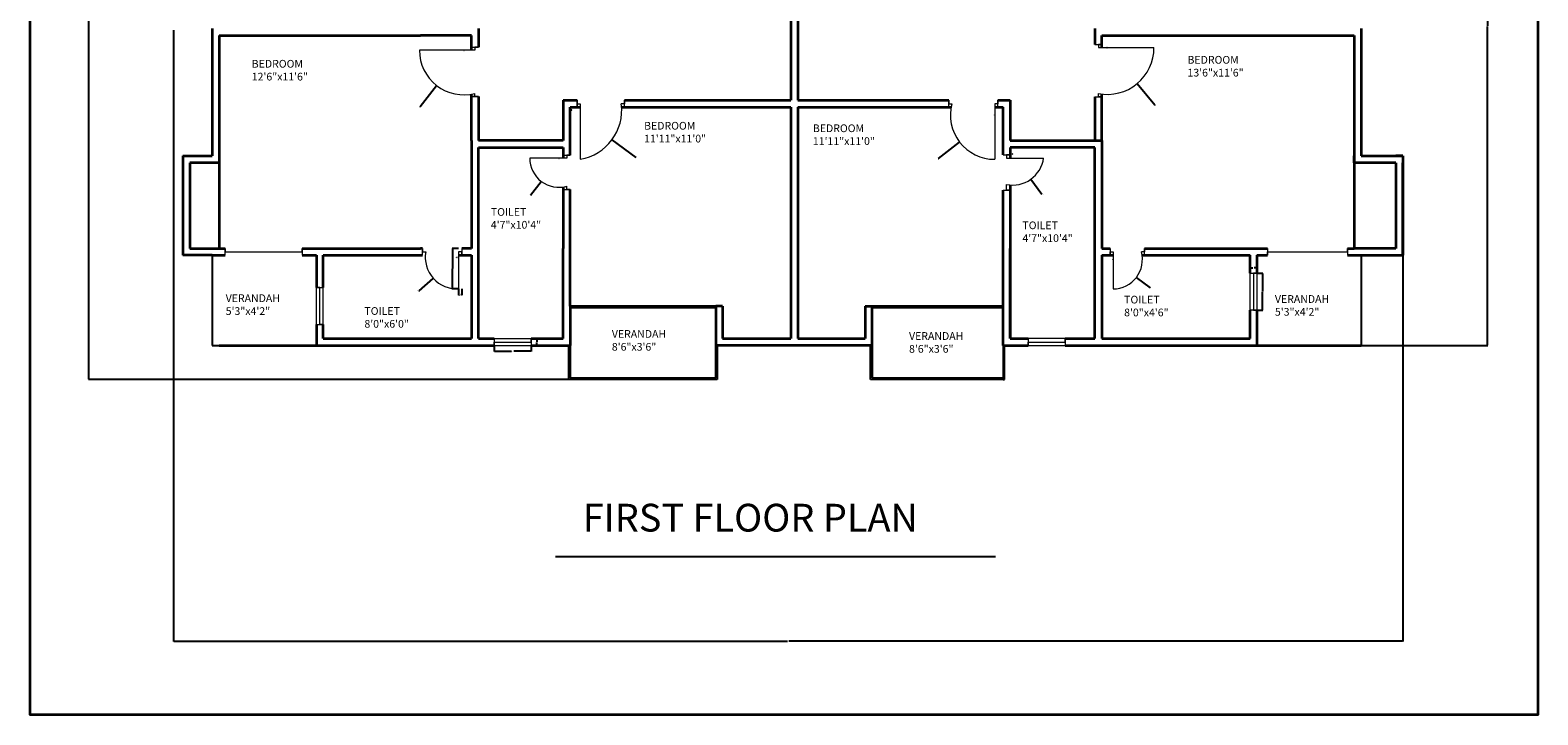
# Model space of a CAD drawing. Units: inches. Extents: x 2154 to 3131, y 1384 to 2688.
# Tile 1 of 5: x 2154 to 3131, y 1384 to 1828. Entities that reach past the tile are written whole.
import ezdxf

# ---------------------------------------------------------------- set-up
doc = ezdxf.new("R2010")
doc.units = ezdxf.units.IN
for name, color, linetype, lineweight in [('A-ANNO-DIMS', 2, 'Continuous', 18), ('A-ANNO-TEXT', 7, 'Continuous', 25), ('A-ANNO-TTLB', 7, 'Continuous', 35), ('A-AREA-IDEN', 7, 'Continuous', 18), ('A-DOOR', 31, 'Continuous', 18), ('A-FLOR-BALC', 130, 'Continuous', 25), ('A-GLAZ', 130, 'Continuous', 18), ('A-WALL', 7, 'Continuous', 35)]:
    doc.layers.add(name, color=color, linetype=linetype, lineweight=lineweight)
doc.styles.get("Standard").update_dxf_attribs({"font": 'arial.ttf'})
doc.dimstyles.get("Standard").update_dxf_attribs({"dimtxt": 0.18, "dimasz": 0.18, "dimexe": 0.18, "dimexo": 0.0625, "dimgap": 0.09, "dimtad": 0, "dimtih": 1, "dimtoh": 1, "dimdec": 4, "dimzin": 0, "dimdsep": 46, "dimtxsty": 'Standard', "dimcen": 0.09, "dimadec": 0, "dimazin": 0, "dimtfac": 1, "dimtdec": 4, "dimtofl": 0, "dimtmove": 0, "dimatfit": 3, "dimfxl": 1, "dimtolj": 1, "dimtzin": 0, "dimarcsym": 0})

# ---------------------------------------------------------------- blocks, each defined once
blk = doc.blocks.new('DOOR-LEAF-24-JAMB-A')
for p, q in [((0, 2.25), (0, 26.25)), ((2, 2.25), (0, 2.25)), ((2, 4.5), (2, 0)), ((2, 0), (2, 2.25))]:
    blk.add_line(p, q)
blk = doc.blocks.new('DOOR-LEAF-36-JAMB-A')
for p, q in [((2, 2.25), (2, 38.25)), ((0, 4.5), (0, 0)), ((0, 0), (0, 2.25)), ((0, 2.25), (2, 2.25))]:
    blk.add_line(p, q)
blk = doc.blocks.new('DOOR-LEAF-24-JAMB-B')
for p, q in [((0, 2), (4.5, 2)), ((4.5, 2), (2.25, 2)), ((2.25, 2), (2.25, 0)), ((2.25, 0), (26.25, 0))]:
    blk.add_line(p, q)
blk = doc.blocks.new('DOOR-LEAF-36-JAMB-B')
for p, q in [((2.25, 0), (2.25, 2)), ((2.25, 2), (38.25, 2)), ((0, 0), (4.5, 0)), ((4.5, 0), (2.25, 0))]:
    blk.add_line(p, q)
blk = doc.blocks.new('WIN-24-FRAME-A')
for p, q in [((0, 4.5), (0, 0)), ((0, 4.5), (24, 4.5)), ((0, 0), (0, 2.25)), ((0, 2.25), (24, 2.25)), ((0, 0), (24, 0)), ((24, 2.25), (24, 4.5)), ((24, 4.5), (24, 0))]:
    blk.add_line(p, q)
blk = doc.blocks.new('WIN-24-FRAME-B')
for p, q in [((0, 0), (0, 4.5)), ((0, 4.5), (24, 4.5)), ((24, 2.25), (0, 2.25)), ((0, 2.25), (0, 0)), ((24, 4.5), (24, 0)), ((24, 0), (24, 2.25)), ((24, 0), (0, 0))]:
    blk.add_line(p, q)
blk = doc.blocks.new('*D10')
at = {"layer": 'A-ANNO-DIMS', "color": 0, "lineweight": -2, "transparency": 16777216}
for p, q in [((2431.78, 1686.18), (2427.73, 1686.18)), ((2427.91, 1686), (2427.91, 1673.23)), ((2427.91, 1660.11), (2427.91, 1672.87)), ((2431.78, 1659.93), (2427.73, 1659.93))]:
    blk.add_line(p, q, dxfattribs=at)
at = {"layer": 'A-ANNO-DIMS', "color": 0, "transparency": 16777216}
for points in [[(2427.88, 1686), (2427.94, 1686), (2427.91, 1686.18)], [(2427.88, 1660.11), (2427.94, 1660.11), (2427.91, 1659.93)]]:
    blk.add_solid(points, dxfattribs=at)
at = {"layer": 'Defpoints', "color": 0, "transparency": 16777216}
for p in [(2431.84, 1686.18), (2427.91, 1659.93), (2431.84, 1659.93)]:
    blk.add_point(p, dxfattribs=at)
at = {"layer": 'A-ANNO-DIMS', "color": 0, "transparency": 16777216, "insert": (2427.91, 1673.05), "char_height": 0.18, "attachment_point": 5}
blk.add_mtext('\\A1;D2 26 TYP.', dxfattribs=at)
blk = doc.blocks.new('*D11')
at = {"layer": 'A-ANNO-DIMS', "color": 0, "lineweight": -2, "transparency": 16777216}
for p, q in [((2431.84, 1659.86), (2431.84, 1655.81)), ((2432.02, 1655.99), (2432.38, 1655.99)), ((2433.66, 1655.99), (2433.3, 1655.99)), ((2433.84, 1659.86), (2433.84, 1655.81))]:
    blk.add_line(p, q, dxfattribs=at)
at = {"layer": 'A-ANNO-DIMS', "color": 0, "transparency": 16777216}
for points in [[(2432.02, 1656.02), (2432.02, 1655.96), (2431.84, 1655.99)], [(2433.66, 1656.02), (2433.66, 1655.96), (2433.84, 1655.99)]]:
    blk.add_solid(points, dxfattribs=at)
at = {"layer": 'Defpoints', "color": 0, "transparency": 16777216}
for p in [(2431.84, 1659.93), (2433.84, 1659.93), (2433.84, 1655.99)]:
    blk.add_point(p, dxfattribs=at)
at = {"layer": 'A-ANNO-DIMS', "color": 0, "transparency": 16777216, "insert": (2432.84, 1655.99), "char_height": 0.18, "attachment_point": 5}
blk.add_mtext('\\A1;2 TYP.', dxfattribs=at)
blk = doc.blocks.new('*D16')
at = {"layer": 'A-ANNO-DIMS', "color": 0, "lineweight": -2, "transparency": 16777216}
for p, q in [((2454.9, 1623.11), (2454.9, 1619.4)), ((2478.9, 1623.11), (2478.9, 1619.4)), ((2455.08, 1619.58), (2466.14, 1619.58)), ((2478.72, 1619.58), (2467.65, 1619.58))]:
    blk.add_line(p, q, dxfattribs=at)
at = {"layer": 'A-ANNO-DIMS', "color": 0, "transparency": 16777216}
for points in [[(2455.08, 1619.61), (2455.08, 1619.55), (2454.9, 1619.58)], [(2478.72, 1619.61), (2478.72, 1619.55), (2478.9, 1619.58)]]:
    blk.add_solid(points, dxfattribs=at)
at = {"layer": 'Defpoints', "color": 0, "transparency": 16777216}
for p in [(2454.9, 1623.18), (2478.9, 1623.18), (2478.9, 1619.58)]:
    blk.add_point(p, dxfattribs=at)
at = {"layer": 'A-ANNO-DIMS', "color": 0, "transparency": 16777216, "insert": (2466.9, 1619.58), "char_height": 0.18, "attachment_point": 5}
blk.add_mtext('\\A1;W1 24 TYP.', dxfattribs=at)
blk = doc.blocks.new('*D17')
at = {"layer": 'A-ANNO-DIMS', "color": 0, "lineweight": -2, "transparency": 16777216}
for p, q in [((2478.96, 1627.68), (2482.68, 1627.68)), ((2478.96, 1623.18), (2482.68, 1623.18)), ((2482.5, 1627.5), (2482.5, 1625.61)), ((2482.5, 1623.36), (2482.5, 1625.25))]:
    blk.add_line(p, q, dxfattribs=at)
at = {"layer": 'A-ANNO-DIMS', "color": 0, "transparency": 16777216}
for points in [[(2482.47, 1627.5), (2482.53, 1627.5), (2482.5, 1627.68)], [(2482.47, 1623.36), (2482.53, 1623.36), (2482.5, 1623.18)]]:
    blk.add_solid(points, dxfattribs=at)
at = {"layer": 'Defpoints', "color": 0, "transparency": 16777216}
for p in [(2478.9, 1627.68), (2478.9, 1623.18), (2482.5, 1627.68)]:
    blk.add_point(p, dxfattribs=at)
at = {"layer": 'A-ANNO-DIMS', "color": 0, "transparency": 16777216, "insert": (2482.5, 1625.43), "char_height": 0.18, "attachment_point": 5}
blk.add_mtext('\\A1;5 TYP.', dxfattribs=at)
blk = doc.blocks.new('*D18')
at = {"layer": 'A-ANNO-DIMS', "color": 0, "lineweight": -2, "transparency": 16777216}
for p, q in [((2949.22, 1670.02), (2952.94, 1670.02)), ((2952.76, 1669.84), (2952.76, 1658.2)), ((2952.76, 1646.2), (2952.76, 1657.84)), ((2949.22, 1646.02), (2952.94, 1646.02))]:
    blk.add_line(p, q, dxfattribs=at)
at = {"layer": 'A-ANNO-DIMS', "color": 0, "transparency": 16777216}
for points in [[(2952.73, 1669.84), (2952.79, 1669.84), (2952.76, 1670.02)], [(2952.73, 1646.2), (2952.79, 1646.2), (2952.76, 1646.02)]]:
    blk.add_solid(points, dxfattribs=at)
at = {"layer": 'Defpoints', "color": 0, "transparency": 16777216}
for p in [(2949.16, 1670.02), (2952.76, 1670.02), (2949.16, 1646.02)]:
    blk.add_point(p, dxfattribs=at)
at = {"layer": 'A-ANNO-DIMS', "color": 0, "transparency": 16777216, "insert": (2952.76, 1658.02), "char_height": 0.18, "attachment_point": 5}
blk.add_mtext('\\A1;W2 24 TYP.', dxfattribs=at)
blk = doc.blocks.new('*D19')
at = {"layer": 'A-ANNO-DIMS', "color": 0, "lineweight": -2, "transparency": 16777216}
for p, q in [((2944.66, 1670.08), (2944.66, 1673.8)), ((2944.84, 1673.62), (2946.45, 1673.62)), ((2948.98, 1673.62), (2947.36, 1673.62)), ((2949.16, 1670.08), (2949.16, 1673.8))]:
    blk.add_line(p, q, dxfattribs=at)
at = {"layer": 'A-ANNO-DIMS', "color": 0, "transparency": 16777216}
for points in [[(2944.84, 1673.65), (2944.84, 1673.59), (2944.66, 1673.62)], [(2948.98, 1673.65), (2948.98, 1673.59), (2949.16, 1673.62)]]:
    blk.add_solid(points, dxfattribs=at)
at = {"layer": 'Defpoints', "color": 0, "transparency": 16777216}
for p in [(2944.66, 1673.62), (2944.66, 1670.02), (2949.16, 1670.02)]:
    blk.add_point(p, dxfattribs=at)
at = {"layer": 'A-ANNO-DIMS', "color": 0, "transparency": 16777216, "insert": (2946.91, 1673.62), "char_height": 0.18, "attachment_point": 5}
blk.add_mtext('\\A1;5 TYP.', dxfattribs=at)
blk = doc.blocks.new('*D22')
at = {"layer": 'A-ANNO-DIMS', "color": 0, "lineweight": -2, "transparency": 16777216}
for p, q in [((2247.16, 1827.61), (2247.16, 1431.24)), ((3043.66, 1681.61), (3043.66, 1431.24)), ((2247.34, 1431.42), (2645.01, 1431.42)), ((3043.48, 1431.42), (2645.8, 1431.42))]:
    blk.add_line(p, q, dxfattribs=at)
at = {"layer": 'A-ANNO-DIMS', "color": 0, "transparency": 16777216}
for points in [[(2247.34, 1431.45), (2247.34, 1431.39), (2247.16, 1431.42)], [(3043.48, 1431.45), (3043.48, 1431.39), (3043.66, 1431.42)]]:
    blk.add_solid(points, dxfattribs=at)
at = {"layer": 'Defpoints', "color": 0, "transparency": 16777216}
for p in [(2247.16, 1827.68), (3043.66, 1681.68), (3043.66, 1431.42)]:
    blk.add_point(p, dxfattribs=at)
at = {"layer": 'A-ANNO-DIMS', "color": 0, "transparency": 16777216, "insert": (2645.41, 1431.42), "char_height": 0.18, "attachment_point": 5}
blk.add_mtext('\\A1;796.5', dxfattribs=at)
blk = doc.blocks.new('*D23')
at = {"layer": 'A-ANNO-DIMS', "color": 0, "lineweight": -2, "transparency": 16777216}
for p, q in [((2504.09, 2580.68), (2192.08, 2580.68)), ((2192.26, 2580.5), (2192.26, 2091.11)), ((2192.26, 1601.36), (2192.26, 2090.74)), ((2504.09, 1601.18), (2192.08, 1601.18))]:
    blk.add_line(p, q, dxfattribs=at)
at = {"layer": 'A-ANNO-DIMS', "color": 0, "transparency": 16777216}
for points in [[(2192.23, 2580.5), (2192.29, 2580.5), (2192.26, 2580.68)], [(2192.23, 1601.36), (2192.29, 1601.36), (2192.26, 1601.18)]]:
    blk.add_solid(points, dxfattribs=at)
at = {"layer": 'Defpoints', "color": 0, "transparency": 16777216}
for p in [(2192.26, 2580.68), (2504.16, 2580.68), (2504.16, 1601.18)]:
    blk.add_point(p, dxfattribs=at)
at = {"layer": 'A-ANNO-DIMS', "color": 0, "transparency": 16777216, "insert": (2192.26, 2090.93), "char_height": 0.18, "attachment_point": 5}
blk.add_mtext('\\A1;979.5', dxfattribs=at)
blk = doc.blocks.new('*D30')
at = {"layer": 'A-ANNO-DIMS', "color": 0, "lineweight": -2, "transparency": 16777216}
for p, q in [((3012.22, 2037.18), (3098.74, 2037.18)), ((3098.56, 2037), (3098.56, 1830.36)), ((3098.56, 1623.36), (3098.56, 1830)), ((3016.72, 1623.18), (3098.74, 1623.18))]:
    blk.add_line(p, q, dxfattribs=at)
at = {"layer": 'A-ANNO-DIMS', "color": 0, "transparency": 16777216}
for points in [[(3098.53, 2037), (3098.59, 2037), (3098.56, 2037.18)], [(3098.53, 1623.36), (3098.59, 1623.36), (3098.56, 1623.18)]]:
    blk.add_solid(points, dxfattribs=at)
at = {"layer": 'Defpoints', "color": 0, "transparency": 16777216}
for p in [(3012.16, 2037.18), (3098.56, 2037.18), (3016.66, 1623.18)]:
    blk.add_point(p, dxfattribs=at)
at = {"layer": 'A-ANNO-DIMS', "color": 0, "transparency": 16777216, "insert": (3098.56, 1830.18), "char_height": 0.18, "attachment_point": 5}
blk.add_mtext('\\A1;414', dxfattribs=at)
blk = doc.blocks.new('*D37')
at = {"layer": 'A-ANNO-DIMS', "color": 0, "lineweight": -2, "transparency": 16777216}
for p, q in [((2504.99, 1775.9), (2505.17, 1775.9)), ((2505.08, 1775.81), (2505.08, 1775.99)), ((2546.79, 1745.01), (2531.3, 1756.48)), ((2546.97, 1745.01), (2546.79, 1745.01))]:
    blk.add_line(p, q, dxfattribs=at)
at = {"layer": 'A-ANNO-DIMS', "color": 0, "transparency": 16777216}
blk.add_solid([(2531.31, 1756.51), (2531.28, 1756.46), (2531.15, 1756.59)], dxfattribs=at)
at = {"layer": 'Defpoints', "color": 0, "transparency": 16777216}
for p in [(2505.08, 1775.9), (2531.15, 1756.59)]:
    blk.add_point(p, dxfattribs=at)
at = {"layer": 'A-ANNO-DIMS', "color": 0, "transparency": 16777216, "insert": (2547.45, 1745.01), "char_height": 0.18, "attachment_point": 5}
blk.add_mtext('\\A1;R32.44', dxfattribs=at)
blk = doc.blocks.new('*D39')
at = {"layer": 'A-ANNO-DIMS', "color": 0, "lineweight": -2, "transparency": 16777216}
for p, q in [((2851.92, 1816.37), (2852.1, 1816.37)), ((2852.01, 1816.28), (2852.01, 1816.46)), ((2883.06, 1778.95), (2871.54, 1792.84)), ((2883.24, 1778.95), (2883.06, 1778.95))]:
    blk.add_line(p, q, dxfattribs=at)
at = {"layer": 'A-ANNO-DIMS', "color": 0, "transparency": 16777216}
blk.add_solid([(2871.56, 1792.86), (2871.51, 1792.82), (2871.42, 1792.98)], dxfattribs=at)
at = {"layer": 'Defpoints', "color": 0, "transparency": 16777216}
for p in [(2852.01, 1816.37), (2871.42, 1792.98)]:
    blk.add_point(p, dxfattribs=at)
at = {"layer": 'A-ANNO-DIMS', "color": 0, "transparency": 16777216, "insert": (2883.72, 1778.95), "char_height": 0.18, "attachment_point": 5}
blk.add_mtext('\\A1;R30.39', dxfattribs=at)
blk = doc.blocks.new('*D41')
at = {"layer": 'A-ANNO-DIMS', "color": 0, "lineweight": -2, "transparency": 16777216}
for p, q in [((2435.2, 1814.62), (2435.38, 1814.62)), ((2435.29, 1814.53), (2435.29, 1814.71)), ((2406.92, 1778.14), (2417.45, 1791.68)), ((2406.74, 1778.14), (2406.92, 1778.14))]:
    blk.add_line(p, q, dxfattribs=at)
at = {"layer": 'A-ANNO-DIMS', "color": 0, "transparency": 16777216}
blk.add_solid([(2417.43, 1791.7), (2417.47, 1791.66), (2417.56, 1791.82)], dxfattribs=at)
at = {"layer": 'Defpoints', "color": 0, "transparency": 16777216}
for p in [(2435.29, 1814.62), (2417.56, 1791.82)]:
    blk.add_point(p, dxfattribs=at)
at = {"layer": 'A-ANNO-DIMS', "color": 0, "transparency": 16777216, "insert": (2406.26, 1778.14), "char_height": 0.18, "attachment_point": 5}
blk.add_mtext('\\A1;R28.88', dxfattribs=at)
blk = doc.blocks.new('*D42')
at = {"layer": 'A-ANNO-DIMS', "color": 0, "lineweight": -2, "transparency": 16777216}
for p, q in [((2779.13, 1772.68), (2779.31, 1772.68)), ((2779.22, 1772.59), (2779.22, 1772.77)), ((2742.82, 1744.55), (2756.33, 1754.99)), ((2742.64, 1744.55), (2742.82, 1744.55))]:
    blk.add_line(p, q, dxfattribs=at)
at = {"layer": 'A-ANNO-DIMS', "color": 0, "transparency": 16777216}
blk.add_solid([(2756.31, 1755.01), (2756.35, 1754.97), (2756.47, 1755.1)], dxfattribs=at)
at = {"layer": 'Defpoints', "color": 0, "transparency": 16777216}
for p in [(2779.22, 1772.68), (2756.47, 1755.1)]:
    blk.add_point(p, dxfattribs=at)
at = {"layer": 'A-ANNO-DIMS', "color": 0, "transparency": 16777216, "insert": (2742.09, 1744.55), "char_height": 0.18, "attachment_point": 5}
blk.add_mtext('\\A1;R28.754', dxfattribs=at)
blk = doc.blocks.new('*D53')
at = {"layer": 'A-ANNO-DIMS', "color": 0, "lineweight": -2, "transparency": 16777216}
for p, q in [((2790.74, 1747.45), (2790.92, 1747.45)), ((2790.83, 1747.36), (2790.83, 1747.54)), ((2809.67, 1721.08), (2802.71, 1730.82)), ((2809.85, 1721.08), (2809.67, 1721.08))]:
    blk.add_line(p, q, dxfattribs=at)
at = {"layer": 'A-ANNO-DIMS', "color": 0, "transparency": 16777216}
blk.add_solid([(2802.74, 1730.84), (2802.69, 1730.81), (2802.61, 1730.97)], dxfattribs=at)
at = {"layer": 'Defpoints', "color": 0, "transparency": 16777216}
for p in [(2790.83, 1747.45), (2802.61, 1730.97)]:
    blk.add_point(p, dxfattribs=at)
at = {"layer": 'A-ANNO-DIMS', "color": 0, "transparency": 16777216, "insert": (2810.4, 1721.08), "char_height": 0.18, "attachment_point": 5}
blk.add_mtext('\\A1;R20.257', dxfattribs=at)
blk = doc.blocks.new('*D54')
at = {"layer": 'A-ANNO-DIMS', "color": 0, "lineweight": -2, "transparency": 16777216}
for p, q in [((2430.64, 1680.42), (2430.82, 1680.42)), ((2430.73, 1680.33), (2430.73, 1680.51)), ((2406.19, 1658.61), (2415.26, 1666.67)), ((2406.01, 1658.61), (2406.19, 1658.61))]:
    blk.add_line(p, q, dxfattribs=at)
at = {"layer": 'A-ANNO-DIMS', "color": 0, "transparency": 16777216}
blk.add_solid([(2415.24, 1666.69), (2415.28, 1666.64), (2415.39, 1666.79)], dxfattribs=at)
at = {"layer": 'Defpoints', "color": 0, "transparency": 16777216}
for p in [(2430.73, 1680.42), (2415.39, 1666.79)]:
    blk.add_point(p, dxfattribs=at)
at = {"layer": 'A-ANNO-DIMS', "color": 0, "transparency": 16777216, "insert": (2405.53, 1658.61), "char_height": 0.18, "attachment_point": 5}
blk.add_mtext('\\A1;R20.52', dxfattribs=at)
blk = doc.blocks.new('*D57')
at = {"layer": 'A-ANNO-DIMS', "color": 0, "lineweight": -2, "transparency": 16777216}
for p, q in [((2855.85, 1678.89), (2856.03, 1678.89)), ((2855.94, 1678.8), (2855.94, 1678.98)), ((2880.08, 1660.5), (2871.17, 1667.29)), ((2880.26, 1660.5), (2880.08, 1660.5))]:
    blk.add_line(p, q, dxfattribs=at)
at = {"layer": 'A-ANNO-DIMS', "color": 0, "transparency": 16777216}
blk.add_solid([(2871.19, 1667.31), (2871.16, 1667.27), (2871.03, 1667.4)], dxfattribs=at)
at = {"layer": 'Defpoints', "color": 0, "transparency": 16777216}
for p in [(2855.94, 1678.89), (2871.03, 1667.4)]:
    blk.add_point(p, dxfattribs=at)
at = {"layer": 'A-ANNO-DIMS', "color": 0, "transparency": 16777216, "insert": (2880.81, 1660.5), "char_height": 0.18, "attachment_point": 5}
blk.add_mtext('\\A1;R18.968', dxfattribs=at)
blk = doc.blocks.new('*D58')
at = {"layer": 'A-ANNO-DIMS', "color": 0, "lineweight": -2, "transparency": 16777216}
for p, q in [((2496.78, 1744.71), (2496.96, 1744.71)), ((2496.87, 1744.62), (2496.87, 1744.8)), ((2478.49, 1720.58), (2485.27, 1729.49)), ((2478.31, 1720.58), (2478.49, 1720.58))]:
    blk.add_line(p, q, dxfattribs=at)
at = {"layer": 'A-ANNO-DIMS', "color": 0, "transparency": 16777216}
blk.add_solid([(2485.25, 1729.5), (2485.29, 1729.47), (2485.38, 1729.63)], dxfattribs=at)
at = {"layer": 'Defpoints', "color": 0, "transparency": 16777216}
for p in [(2496.87, 1744.71), (2485.38, 1729.63)]:
    blk.add_point(p, dxfattribs=at)
at = {"layer": 'A-ANNO-DIMS', "color": 0, "transparency": 16777216, "insert": (2477.83, 1720.58), "char_height": 0.18, "attachment_point": 5}
blk.add_mtext('\\A1;R18.96', dxfattribs=at)

msp = doc.modelspace()

# ---------------------------------------------------------------- linework, layer by layer
at = {"layer": 'A-ANNO-TEXT'}
msp.add_line((2494.5533, 1486.3159), (2779.6429, 1486.3159), dxfattribs=at)
at = {"layer": 'A-ANNO-TTLB'}
msp.add_lwpolyline([(2154.1953, 2688.4009), (3131.1627, 2688.4009), (3131.1627, 1383.7377), (2154.1953, 1383.7377)], close=True, dxfattribs=at)
at = {"layer": 'A-DOOR'}
for p, q in [((2442.406, 1816.6226), (2442.406, 1816.6226)), ((2440.156, 1784.6331), (2444.656, 1784.6331)), ((2444.656, 1784.6331), (2440.156, 1784.6331)), ((2440.156, 1784.6331), (2442.406, 1784.6331)), ((2442.406, 1784.6331), (2442.406, 1786.6331)), ((2508.61, 1778.9333), (2508.61, 1782.1799)), ((2508.61, 1779.9299), (2508.61, 1779.9299)), ((2539.27, 1779.9299), (2537.27, 1779.9299)), ((2539.27, 1777.6799), (2539.27, 1782.1799)), ((2539.27, 1782.1799), (2539.27, 1779.9299)), ((2749.3955, 1777.6799), (2749.3955, 1782.1799)), ((2749.3955, 1782.1799), (2749.3955, 1779.9299)), ((2749.3955, 1779.9299), (2751.3955, 1779.9299)), ((2844.156, 1784.4983), (2848.656, 1784.4983)), ((2846.406, 1784.4983), (2846.406, 1786.4983)), ((2848.656, 1784.4983), (2846.406, 1784.4983)), ((2499.656, 1724.4345), (2504.156, 1724.4345)), ((2501.906, 1724.4345), (2501.906, 1726.4345)), ((2504.156, 1724.4345), (2501.906, 1724.4345)), ((2784.656, 1724.0013), (2789.156, 1724.0013)), ((2786.906, 1725.5813), (2786.906, 1727.5813)), ((2786.906, 1724.0013), (2786.906, 1725.5813)), ((2789.156, 1724.0013), (2786.906, 1724.0013)), ((2408.5121, 1681.6767), (2408.5121, 1686.1767)), ((2408.5121, 1686.1767), (2408.5121, 1683.9267)), ((2408.5121, 1683.9267), (2410.5121, 1683.9267)), ((2876.2329, 1683.9267), (2874.2329, 1683.9267)), ((2876.1528, 1681.6767), (2876.2329, 1681.6767)), ((2876.2329, 1681.6767), (2876.2329, 1686.1767)), ((2876.2329, 1686.1767), (2876.2329, 1683.9267))]:
    msp.add_line(p, q, dxfattribs=at)
for centre, radius, start, end in [((2435.2867, 1814.6226), 28.8807, 180, 284.2708959), ((2852.0139, 1816.3686), 30.3921, 259.3670447, 360), ((2505.0796, 1775.897), 32.442, 279.8150096, 7.140879), ((2779.2216, 1772.6839), 28.7541, 165.4042728, 270), ((2496.8661, 1744.7124), 18.9601, 180, 285.415643), ((2790.8333, 1747.4541), 20.2572, 258.8212578, 352.2621854), ((2430.731, 1680.4177), 20.5211, 170.1542308, 273.1052455), ((2855.9446, 1678.8947), 18.968, 270, 15.3842986)]:
    msp.add_arc(centre, radius, start, end, dxfattribs=at)
at = {"layer": 'A-FLOR-BALC'}
for p, q in [((2272.156, 1681.6767), (2272.156, 1623.1767)), ((3016.656, 1681.6767), (3016.656, 1623.1767)), ((2598.406, 1648.6767), (2504.156, 1648.6767)), ((2598.406, 1647.6767), (2504.156, 1647.6767)), ((2598.406, 1648.6767), (2598.406, 1647.6767)), ((2598.406, 1648.6767), (2598.406, 1647.6767)), ((2784.656, 1648.6767), (2699.7402, 1648.6767)), ((2784.656, 1647.6767), (2699.7402, 1647.6767)), ((2272.156, 1623.1767), (2276.656, 1623.1767)), ((2503.156, 1601.1767), (2503.156, 1623.1767)), ((2504.156, 1623.1767), (2504.156, 1605.1767)), ((2598.406, 1602.1767), (2598.406, 1623.1767)), ((2598.406, 1623.1767), (2598.406, 1623.1767)), ((2598.406, 1623.1767), (2599.406, 1623.1767)), ((2599.406, 1623.1767), (2599.406, 1602.1767)), ((2698.7402, 1601.1767), (2698.7402, 1623.1767)), ((2699.7402, 1623.1767), (2699.7402, 1605.1767)), ((2784.656, 1623.1767), (2784.656, 1602.1767)), ((2785.656, 1601.1767), (2785.656, 1623.1767)), ((2949.156, 1623.1767), (2944.656, 1623.1767)), ((2504.156, 1605.1767), (2504.156, 1602.1767)), ((2699.7402, 1605.1767), (2699.7402, 1602.1767)), ((2504.156, 1601.1767), (2503.156, 1601.1767)), ((2504.156, 1602.1767), (2598.406, 1602.1767)), ((2599.406, 1601.1767), (2504.156, 1601.1767)), ((2599.406, 1602.1767), (2599.406, 1601.1767)), ((2699.7402, 1601.1767), (2698.7402, 1601.1767)), ((2699.7402, 1602.1767), (2784.656, 1602.1767)), ((2785.656, 1601.1767), (2699.7402, 1601.1767)), ((2784.656, 1601.1767), (2785.656, 1601.1767))]:
    msp.add_line(p, q, dxfattribs=at)
at = {"layer": 'A-GLAZ'}
for p, q in [((2280.5517, 1681.6767), (2280.5517, 1686.1767)), ((2280.5517, 1686.1767), (2280.5517, 1683.9267)), ((2280.5517, 1683.9267), (2330.3831, 1683.9267)), ((2330.3831, 1683.9267), (2330.3831, 1686.1767)), ((2330.3831, 1686.1767), (2330.3831, 1681.6767)), ((2955.9275, 1686.1767), (2955.9275, 1681.6767)), ((2955.9275, 1681.6767), (2955.9275, 1683.9267)), ((2955.9275, 1683.9267), (2955.9275, 1683.9267)), ((2955.9275, 1683.9267), (3007.8885, 1683.9267)), ((3007.8885, 1683.9267), (3007.8885, 1686.1767)), ((3007.8885, 1686.1767), (3007.8885, 1681.6767)), ((2454.8984, 1625.4267), (2454.8984, 1625.4267)), ((2800.9225, 1627.6767), (2800.9225, 1624.4228)), ((2824.9225, 1627.6767), (2800.9225, 1627.6767)), ((2800.9225, 1623.1767), (2800.9225, 1625.4724)), ((2800.9225, 1625.4724), (2824.9225, 1625.4724)), ((2800.9225, 1624.4228), (2800.9225, 1623.1767)), ((2800.9225, 1623.1767), (2824.9225, 1623.1767)), ((2824.9225, 1625.4724), (2824.9225, 1627.6767)), ((2824.9225, 1627.6767), (2824.9225, 1623.1767))]:
    msp.add_line(p, q, dxfattribs=at)
at = {"layer": 'A-WALL'}
for p, q in [((2647.156, 2037.1767), (2647.156, 1782.1799)), ((2651.656, 2037.1767), (2651.656, 1782.1799)), ((2272.156, 1828.6767), (2272.156, 1746.1767)), ((2444.656, 1828.6767), (2444.656, 1816.6226)), ((2844.156, 1828.6767), (2844.156, 1818.3686)), ((3016.656, 1828.6767), (3016.656, 1746.1767)), ((2276.656, 1824.1767), (2407.156, 1824.1767)), ((2276.656, 1824.1767), (2276.656, 1741.6767)), ((2440.156, 1824.1767), (2407.156, 1824.1767)), ((2440.156, 1814.6226), (2440.156, 1824.1767)), ((2848.656, 1824.1767), (2873.0368, 1824.1767)), ((2848.656, 1816.3686), (2848.656, 1824.1767)), ((2873.0368, 1824.1767), (3012.156, 1824.1767)), ((3012.156, 1824.1767), (3012.156, 1741.6767)), ((2440.156, 1756.1767), (2440.156, 1786.1554)), ((2444.656, 1784.6331), (2444.656, 1756.1767)), ((2499.656, 1782.1799), (2499.656, 1756.1767)), ((2499.656, 1782.1799), (2508.61, 1782.1799)), ((2539.27, 1782.1799), (2647.156, 1782.1799)), ((2651.656, 1782.1799), (2749.3955, 1782.1799)), ((2781.2216, 1782.1799), (2789.156, 1782.1799)), ((2789.156, 1782.1799), (2789.156, 1756.1767)), ((2844.156, 1784.4983), (2844.156, 1756.1767)), ((2848.656, 1756.1767), (2848.656, 1786.1625)), ((2504.156, 1777.6799), (2510.61, 1777.6799)), ((2504.156, 1746.7124), (2504.156, 1777.6799)), ((2537.4726, 1777.6799), (2647.156, 1777.6799)), ((2647.156, 1777.6799), (2647.156, 1627.6767)), ((2651.656, 1777.6799), (2750.9049, 1777.6799)), ((2651.656, 1777.6799), (2651.656, 1627.6767)), ((2779.2216, 1777.6799), (2784.656, 1777.6799)), ((2784.656, 1746.7267), (2784.656, 1777.6799)), ((2440.156, 1756.1767), (2440.156, 1686.1767)), ((2499.656, 1756.1767), (2444.656, 1756.1767)), ((2444.656, 1627.6767), (2444.656, 1751.6767)), ((2444.656, 1751.6767), (2499.656, 1751.6767)), ((2499.656, 1751.6767), (2499.656, 1744.7124)), ((2504.156, 1751.6767), (2504.156, 1756.1767)), ((2784.656, 1751.6767), (2784.656, 1756.1767)), ((2789.156, 1756.1767), (2844.156, 1756.1767)), ((2789.156, 1751.6767), (2789.156, 1744.7267)), ((2844.156, 1751.6767), (2789.156, 1751.6767)), ((2844.156, 1756.1767), (2848.656, 1756.1767)), ((2844.156, 1686.1767), (2844.156, 1751.6767)), ((2848.656, 1756.1767), (2848.656, 1686.1767)), ((2253.1496, 1746.1767), (2272.156, 1746.1767)), ((2253.1496, 1746.1767), (2253.1496, 1681.6767)), ((2276.656, 1741.6767), (2257.6496, 1741.6767)), ((2257.6496, 1741.6767), (2257.6496, 1686.1767)), ((2276.656, 1746.1767), (2276.656, 1741.6767)), ((2276.656, 1741.6767), (2276.656, 1686.1767)), ((3012.156, 1741.6767), (3012.156, 1746.1767)), ((3039.156, 1741.6767), (3012.156, 1741.6767)), ((3012.156, 1741.6767), (3012.156, 1686.1767)), ((3016.656, 1746.1767), (3043.656, 1746.1767)), ((3043.656, 1746.1767), (3039.156, 1746.1767)), ((3039.156, 1741.6767), (3039.156, 1686.1767)), ((3043.656, 1746.1767), (3043.656, 1681.6767)), ((3043.656, 1681.6767), (3043.656, 1741.6767)), ((2499.656, 1725.9588), (2499.656, 1686.1767)), ((2504.156, 1686.1767), (2504.156, 1724.4345)), ((2784.656, 1648.6767), (2784.656, 1724.0013)), ((2789.156, 1727.2665), (2789.156, 1627.6767)), ((2272.156, 1681.6767), (2253.1496, 1681.6767)), ((2257.6496, 1686.1767), (2280.5517, 1686.1767)), ((2272.156, 1681.6767), (2280.5517, 1681.6767)), ((2330.3831, 1686.1767), (2407.156, 1686.1767)), ((2330.3831, 1681.6767), (2339.656, 1681.6767)), ((2339.656, 1681.6767), (2339.656, 1660.7286)), ((2344.156, 1660.7286), (2344.156, 1681.6767)), ((2344.156, 1681.6767), (2408.5121, 1681.6767)), ((2408.5121, 1686.1767), (2407.156, 1686.1767)), ((2431.8426, 1681.6767), (2440.156, 1681.6767)), ((2440.156, 1686.1767), (2433.8426, 1686.1767)), ((2440.156, 1681.6767), (2440.156, 1627.6767)), ((2444.656, 1627.6767), (2444.656, 1686.1767)), ((2499.656, 1627.6767), (2499.656, 1686.1767)), ((2504.156, 1648.6767), (2504.156, 1686.1767)), ((2784.656, 1623.1767), (2784.656, 1686.1767)), ((2789.156, 1627.6767), (2789.156, 1686.1767)), ((2844.156, 1627.6767), (2844.156, 1686.1767)), ((2848.656, 1686.1767), (2853.9446, 1686.1767)), ((2848.656, 1681.6767), (2855.9446, 1681.6767)), ((2848.656, 1681.6767), (2848.656, 1627.6767)), ((2874.7075, 1681.6767), (2944.656, 1681.6767)), ((2876.2329, 1686.1767), (2955.9275, 1686.1767)), ((2944.656, 1670.0203), (2944.656, 1681.6767)), ((2949.156, 1681.6767), (2949.156, 1670.0203)), ((2949.156, 1681.6767), (2955.9275, 1681.6767)), ((3007.8885, 1686.1767), (3012.156, 1686.1767)), ((3007.8885, 1681.6767), (3016.656, 1681.6767)), ((3039.156, 1686.1767), (3012.156, 1686.1767)), ((3016.656, 1681.6767), (3043.656, 1681.6767)), ((2504.156, 1648.6767), (2504.156, 1623.1767)), ((2602.906, 1648.6767), (2598.406, 1648.6767)), ((2598.406, 1648.6767), (2598.406, 1623.1767)), ((2602.906, 1648.6767), (2602.906, 1627.6767)), ((2695.2402, 1648.6767), (2695.2402, 1627.6767)), ((2695.2402, 1648.6767), (2699.7402, 1648.6767)), ((2699.7402, 1645.6767), (2699.7402, 1648.6767)), ((2699.7402, 1623.1767), (2699.7402, 1645.6767)), ((2944.656, 1627.6767), (2944.656, 1646.0203)), ((2949.156, 1646.0203), (2949.156, 1623.1767)), ((2339.656, 1636.7286), (2339.656, 1623.1767)), ((2344.156, 1627.6767), (2344.156, 1636.7286)), ((2276.656, 1623.1767), (2454.8984, 1623.1767)), ((2344.156, 1627.6767), (2440.156, 1627.6767)), ((2444.656, 1627.6767), (2454.8984, 1627.6767)), ((2478.8984, 1627.6767), (2499.656, 1627.6767)), ((2478.8984, 1623.1767), (2504.156, 1623.1767)), ((2699.7402, 1623.1767), (2598.406, 1623.1767)), ((2598.406, 1623.1767), (2598.406, 1623.1767)), ((2602.906, 1627.6767), (2647.156, 1627.6767)), ((2651.656, 1627.6767), (2695.2402, 1627.6767)), ((2784.656, 1623.1767), (2800.9225, 1623.1767)), ((2789.156, 1627.6767), (2800.9225, 1627.6767)), ((2824.9225, 1627.6767), (2844.156, 1627.6767)), ((2824.9225, 1623.1767), (3016.656, 1623.1767)), ((2848.656, 1627.6767), (2944.656, 1627.6767))]:
    msp.add_line(p, q, dxfattribs=at)

# ---------------------------------------------------------------- block references
at = {"layer": 'A-DOOR', "extrusion": (0, 0, -1), "zscale": -1}
for name, p, rotation in [('DOOR-LEAF-36-JAMB-B', (-2844.156, 1818.3686), 180), ('DOOR-LEAF-36-JAMB-A', (-2444.656, 1816.6226), 270.0000000000008), ('DOOR-LEAF-24-JAMB-B', (-2855.9446, 1686.1767), 269.9999999999999)]:
    msp.add_blockref(name, p, dxfattribs=dict(at, rotation=rotation))
at = {"layer": 'A-DOOR'}
for name, p, rotation in [('DOOR-LEAF-36-JAMB-B', (2508.61, 1782.1799), 270.0000000000008), ('DOOR-LEAF-36-JAMB-A', (2781.2216, 1782.1799), 180), ('DOOR-LEAF-24-JAMB-A', (2504.156, 1744.7124), 90.00000000000067), ('DOOR-LEAF-24-JAMB-B', (2431.8426, 1686.1767), 269.9999999999999)]:
    msp.add_blockref(name, p, dxfattribs=dict(at, rotation=rotation))
msp.add_blockref('DOOR-LEAF-24-JAMB-B', (2784.656, 1744.7267), dxfattribs=at)
at = {"layer": 'A-GLAZ'}
for name, p, rotation in [('WIN-24-FRAME-B', (2949.156, 1646.0203), 89.9999999999937), ('WIN-24-FRAME-A', (2344.156, 1636.7286), 90.00000000000591)]:
    msp.add_blockref(name, p, dxfattribs=dict(at, rotation=rotation))
msp.add_blockref('WIN-24-FRAME-A', (2454.8984, 1623.1767), dxfattribs=at)

# ---------------------------------------------------------------- texts
at = {"layer": 'A-ANNO-TEXT', "insert": (2512.2681, 1520.5824), "char_height": 18, "attachment_point": 1}
msp.add_mtext_dynamic_manual_height_columns('FIRST FLOOR PLAN ', width=702.488963, gutter_width=12.5, heights=[0], dxfattribs=at)
at = {"layer": 'A-AREA-IDEN', "char_height": 5, "attachment_point": 1}
for s, width, insert in [('BEDROOM\\P12\'6"x11\'6"', 183.388614, (2297.7995, 1808.3648)), ('BEDROOM\\P13\'6"x11\'6"', 223.821939, (2904.1547, 1810.9345)), ('BEDROOM\\P11\'11"x11\'0"', 109.361832, (2552.037, 1768.178)), ('BEDROOM\\P11\'11"x11\'0"', 182.757174, (2661.3988, 1766.5549)), ('TOILET\\P4\'7"x10\'4"', 145.460926, (2452.7233, 1712.311)), ('TOILET\\P4\'7"x10\'4"', 88.510397, (2797.1743, 1703.6229)), ('VERANDAH\\P5\'3"x4\'2"', 123.126483, (2280.9143, 1656.3674)), ('TOILET\\P8\'0"x4\'6"', 125.187017, (2863.0864, 1655.4703)), ('VERANDAH\\P5\'3"x4\'2"', 103.531828, (2960.7863, 1655.8672)), ('TOILET\\P8\'0"x6\'0"', 148.357823, (2370.7944, 1648.0809)), ('VERANDAH\\P8\'6"x3\'6"', 127.045563, (2531.1267, 1633.1941)), ('VERANDAH\\P8\'6"x3\'6"', 127.045563, (2723.7108, 1631.8634))]:
    msp.add_mtext_dynamic_manual_height_columns(s, width=width, gutter_width=12.5, heights=[0], dxfattribs=dict(at, insert=insert))

# ---------------------------------------------------------------- dimensions: what is measured, and where the dimension line sits
at = {"layer": 'A-ANNO-DIMS'}
for base, p1, p2, override, picture, middle in [((2192.256, 2580.6767), (2504.156, 1601.1767), (2504.156, 2580.6767), {"dimdec": 1, "dimlfac": 1, "dimrnd": 0, "dimzin": 0, "dimdsep": 46, "dimlunit": 2}, '*D23', (2192.256, 2090.9267)), ((3098.556, 2037.1767), (3016.656, 1623.1767), (3012.156, 2037.1767), {"dimdec": 0, "dimlfac": 1, "dimrnd": 0, "dimzin": 0, "dimdsep": 46, "dimlunit": 2}, '*D30', (3098.556, 1830.1767))]:
    dim = msp.add_linear_dim(base=base, p1=p1, p2=p2, angle=90, dimstyle='Standard', override=override, dxfattribs=at)
    dim.commit()
    dim.dimension.update_dxf_attribs({"geometry": picture, "text_midpoint": middle})
dim = msp.add_linear_dim(base=(3043.656, 1431.4159), p1=(2247.156, 1827.6767), p2=(3043.656, 1681.6767), dimstyle='Standard', override={"dimdec": 1, "dimlfac": 1, "dimrnd": 0, "dimzin": 0, "dimdsep": 46, "dimlunit": 2}, dxfattribs=at)
dim.commit()
dim.dimension.update_dxf_attribs({"geometry": '*D22', "text_midpoint": (2645.406, 1431.4159)})
for center, mpoint, override, picture, middle in [((2435.2867, 1814.6226), (2417.5601, 1791.8221), {"dimdec": 2, "dimlfac": 1, "dimrnd": 0, "dimzin": 0, "dimdsep": 46, "dimlunit": 2}, '*D41', (2406.2641, 1778.1418)), ((2852.0139, 1816.3686), (2871.4207, 1792.9793), {"dimdec": 2, "dimlfac": 1, "dimrnd": 0, "dimzin": 0, "dimdsep": 46, "dimlunit": 2}, '*D39', (2883.7249, 1778.9458)), ((2505.0796, 1775.897), (2531.1511, 1756.5899), {"dimdec": 2, "dimlfac": 1, "dimrnd": 0, "dimzin": 0, "dimdsep": 46, "dimlunit": 2}, '*D37', (2547.4534, 1745.0057)), ((2779.2216, 1772.6839), (2756.4713, 1755.0993), {"dimdec": 3, "dimlfac": 1, "dimrnd": 0, "dimzin": 0, "dimdsep": 46, "dimlunit": 2}, '*D42', (2742.0918, 1744.5485)), ((2496.8661, 1744.7124), (2485.3787, 1729.6286), {"dimdec": 2, "dimlfac": 1, "dimrnd": 0, "dimzin": 0, "dimdsep": 46, "dimlunit": 2}, '*D58', (2477.8264, 1720.5782)), ((2790.8333, 1747.4541), (2802.6089, 1730.9711), {"dimdec": 3, "dimlfac": 1, "dimrnd": 0, "dimzin": 0, "dimdsep": 46, "dimlunit": 2}, '*D53', (2810.404, 1721.0814)), ((2430.731, 1680.4177), (2415.3923, 1666.7853), {"dimdec": 2, "dimlfac": 1, "dimrnd": 0, "dimzin": 0, "dimdsep": 46, "dimlunit": 2}, '*D54', (2405.5302, 1658.6059)), ((2855.9446, 1678.8947), (2871.0316, 1667.3983), {"dimdec": 3, "dimlfac": 1, "dimrnd": 0, "dimzin": 0, "dimdsep": 46, "dimlunit": 2}, '*D57', (2880.8138, 1660.5005))]:
    dim = msp.add_radius_dim(center=center, mpoint=mpoint, dimstyle='Standard', override=override, dxfattribs=at)
    dim.commit()
    dim.dimension.update_dxf_attribs({"geometry": picture, "text_midpoint": middle, "dimtype": 164})
for base, p1, p2, angle, text, picture, middle in [((2427.9051, 1659.9267), (2431.8426, 1686.1767), (2431.8426, 1659.9267), 270, 'D2 <> TYP.', '*D10', (2427.9051, 1673.0517)), ((2944.6560159305, 1673.6202683761), (2949.1560159305, 1670.0202683761), (2944.6560159305, 1670.0202683761), 180, '<> TYP.', '*D19', (2946.9060159305, 1673.6202683761)), ((2952.756, 1670.0203), (2949.156, 1646.0203), (2949.156, 1670.0203), 90, 'W2 <> TYP.', '*D18', (2952.756, 1658.0203)), ((2482.4983579398, 1627.6766960424), (2478.8983579398, 1623.1766960424), (2478.8983579398, 1627.6766960424), 90, '<> TYP.', '*D17', (2482.4983579398, 1625.4266960424))]:
    dim = msp.add_linear_dim(base=base, p1=p1, p2=p2, angle=angle, text=text, dimstyle='Standard', override={"dimdec": 0, "dimlfac": 1, "dimrnd": 0, "dimzin": 0, "dimdsep": 46, "dimlunit": 2}, dxfattribs=at)
    dim.commit()
    dim.dimension.update_dxf_attribs({"geometry": picture, "text_midpoint": middle})
for base, p1, p2, text, picture, middle in [((2433.8426, 1655.9892), (2431.8426, 1659.9267), (2433.8426, 1659.9267), '<> TYP.', '*D11', (2432.8426, 1655.9892)), ((2478.8984, 1619.5767), (2454.8984, 1623.1767), (2478.8984, 1623.1767), 'W1 <> TYP.', '*D16', (2466.8984, 1619.5767))]:
    dim = msp.add_linear_dim(base=base, p1=p1, p2=p2, text=text, dimstyle='Standard', override={"dimdec": 0, "dimlfac": 1, "dimrnd": 0, "dimzin": 0, "dimdsep": 46, "dimlunit": 2}, dxfattribs=at)
    dim.commit()
    dim.dimension.update_dxf_attribs({"geometry": picture, "text_midpoint": middle})

doc.saveas('drawing.dxf')
